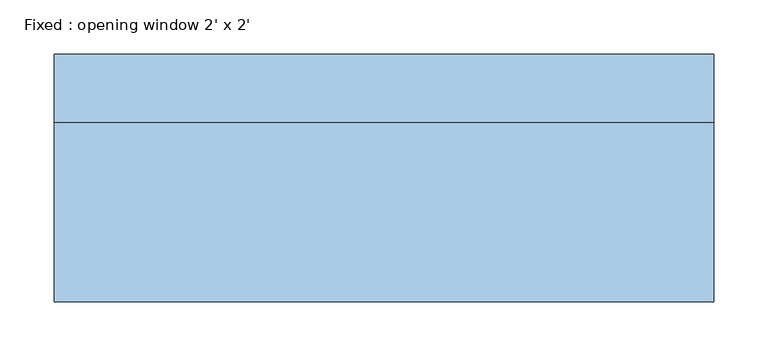
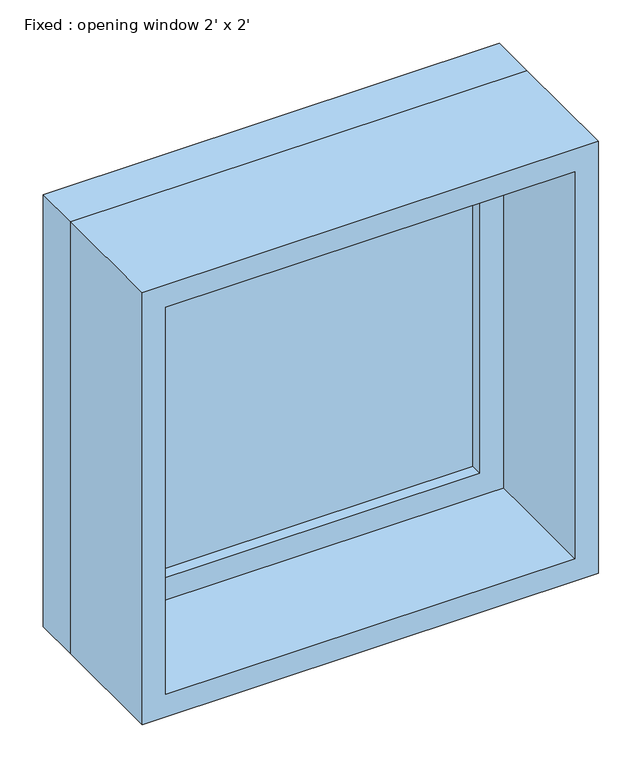
"""IFC4 building model written with IfcOpenShell, lengths in millimetres: window geometry, Fixed : opening window 2' x 2'."""

from ifc_helpers import new_model, si_unit, frame, origin, place, context, project, spatial, polyline, outline, extrude, source, transform, mapped, element, save


def fixed_opening_window_2_x_2_e119d648(model_context):
    return source(origin(), model_context, "Body", "SweptSolid", [
        extrude(outline(polyline([(203.2, 66.675), (-279.4, 66.675), (-279.4, 79.375), (203.2, 79.375), (203.2, 66.675)])), frame((0.0, 0.0, 2197.1), z_axis=(0.0, 0.0, 1.0), x_axis=(1.0, 0.0, 0.0)), (0.0, 0.0, 1.0), 482.6),
        extrude(outline(polyline([(2724.15, -323.85), (2152.65, -323.85), (2152.65, 247.65), (2724.15, 247.65), (2724.15, -323.85)]), holes=[polyline([(2679.7, -279.4), (2679.7, 203.2), (2197.1, 203.2), (2197.1, -279.4), (2679.7, -279.4)])]), frame((0.0, 50.8, 0.0), z_axis=(0.0, 1.0, 0.0), x_axis=(0.0, 0.0, 1.0)), (0.0, 0.0, 1.0), 44.45),
        extrude(outline(polyline([(2743.2, -342.9), (2133.6, -342.9), (2133.6, 266.7), (2743.2, 266.7), (2743.2, -342.9)]), holes=[polyline([(2711.45, -311.15), (2711.45, 234.95), (2165.35, 234.95), (2165.35, -311.15), (2711.45, -311.15)])]), frame((0.0, -114.3, 0.0), z_axis=(0.0, 1.0, 0.0), x_axis=(0.0, 0.0, 1.0)), (0.0, 0.0, 1.0), 165.1),
        extrude(outline(polyline([(2743.2, 266.7), (2743.2, -342.9), (2133.6, -342.9), (2133.6, 266.7), (2743.2, 266.7)]), holes=[polyline([(2724.15, 247.65), (2152.65, 247.65), (2152.65, -323.85), (2724.15, -323.85), (2724.15, 247.65)])]), frame((0.0, 50.8, 0.0), z_axis=(0.0, 1.0, 0.0), x_axis=(0.0, 0.0, 1.0)), (0.0, 0.0, 1.0), 63.5),
    ])


if __name__ == "__main__":
    model = new_model("IFC4")
    model_context = context("Model", 3, world=origin())
    ifc_project = project(units=[si_unit("LENGTHUNIT", "METRE", prefix="MILLI")], contexts=[model_context])
    site = spatial("IfcSite", under=ifc_project)
    building = spatial("IfcBuilding", under=site)
    placement = place(None, origin())
    fixed_opening_window_2_x_2_shape = fixed_opening_window_2_x_2_e119d648(model_context)
    element("IfcWindow", 1, ObjectType="Fixed : opening window 2' x 2'", at=placement, inside=building, context=model_context, shape_type="MappedRepresentation", body=[
        mapped(fixed_opening_window_2_x_2_shape, transform((0.0, 0.0, 0.0), x_axis=(1.0, 0.0, 0.0), y_axis=(0.0, 1.0, 0.0), z_axis=(0.0, 0.0, 1.0))),
    ])
    save(model, "model.ifc")

# Revit data of these elements
# Type "Fixed : opening window 2' x 2'"
#   Type Mark = "18"
#   Construction Type Id = "GSP4R"
#   Assembly Code = "B2020100"
#   Analytic Construction = "1/8 in Pilkington single glazing"
#   Visual Light Transmittance = 0.9
#   Solar Heat Gain Coefficient = 0.78
#   Heat Transfer Coefficient (U) = 0.6496 BTU/(h·ft²·°F)
#   Height = 2' - 0"
#   Default Sill Height = 7' - 0"
#   Width = 2' - 0"
#   Window Inset = 0' - 0 3/4"
#   Define Thermal Properties by = 1
#   Glass Pane Material = Glass
#   Sash Material = Sash
#   Wall Closure = (empty or 0)
# Element 1 (IfcWindow, "Fixed : opening window 2' x 2'")
#   Materials on its faces: "Sash", "Glass"
# Materials
#   "Glass": class "Glass", colour RGB 0 128 192, transparency 0.75, Description = "Soda Lime Glass", Cost = 0
#   "Sash": class "Wood", colour RGB 224 178 126, transparency 0, Cost = 0
